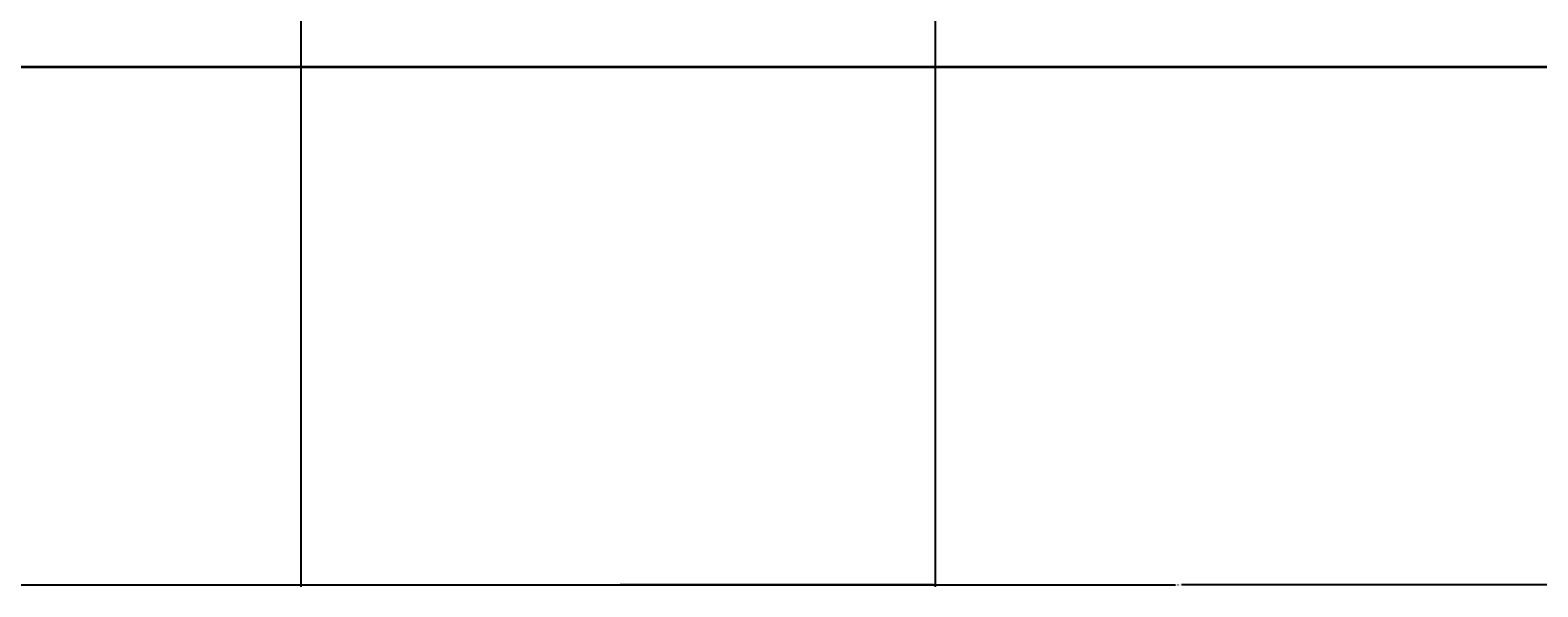
# Model space of a CAD drawing. Units: inches. Extents: x 3731 to 4318, y 1310 to 2388.
# Tile 8 of 57: x 3944 to 4086, y 1310 to 1363. Entities that reach past the tile are written whole.
import ezdxf

# ---------------------------------------------------------------- set-up
doc = ezdxf.new("R2010")
doc.units = ezdxf.units.IN
doc.layers.add('A-ANNO-DIMS', color=2, linetype='Continuous', lineweight=18)
doc.layers.add('A-WALL', color=7, linetype='Continuous', lineweight=35)
doc.styles.get("Standard").update_dxf_attribs({"font": 'arial.ttf'})
doc.dimstyles.get("Standard").update_dxf_attribs({"dimtxt": 0.18, "dimasz": 0.18, "dimexe": 0.18, "dimexo": 0.0625, "dimgap": 0.09, "dimtad": 0, "dimtih": 1, "dimtoh": 1, "dimdec": 4, "dimzin": 0, "dimdsep": 46, "dimtxsty": 'Standard', "dimcen": 0.09, "dimadec": 0, "dimazin": 0, "dimtfac": 1, "dimtdec": 4, "dimtofl": 0, "dimtmove": 0, "dimatfit": 3, "dimfxl": 1, "dimtolj": 1, "dimtzin": 0, "dimarcsym": 0})

# ---------------------------------------------------------------- blocks, each defined once
blk = doc.blocks.new('*D32')
at = {"layer": 'A-ANNO-DIMS', "color": 0, "lineweight": -2, "transparency": 16777216}
for p, q in [((4269.21, 1592.32), (4269.21, 1310.25)), ((3835.21, 1359.32), (3835.21, 1310.25)), ((3835.39, 1310.43), (4051.92, 1310.43)), ((4269.03, 1310.43), (4052.5, 1310.43))]:
    blk.add_line(p, q, dxfattribs=at)
at = {"layer": 'A-ANNO-DIMS', "color": 0, "transparency": 16777216}
for points in [[(3835.39, 1310.46), (3835.39, 1310.4), (3835.21, 1310.43)], [(4269.03, 1310.46), (4269.03, 1310.4), (4269.21, 1310.43)]]:
    blk.add_solid(points, dxfattribs=at)
at = {"layer": 'Defpoints', "color": 0, "transparency": 16777216}
for p in [(4269.21, 1592.38), (3835.21, 1359.38), (4269.21, 1310.43)]:
    blk.add_point(p, dxfattribs=at)
at = {"layer": 'A-ANNO-DIMS', "color": 0, "transparency": 16777216, "insert": (4052.21, 1310.43), "char_height": 0.18, "attachment_point": 5}
blk.add_mtext('\\A1;434', dxfattribs=at)
blk = doc.blocks.new('*D44')
at = {"layer": 'A-ANNO-DIMS', "color": 0, "lineweight": -2, "transparency": 16777216}
for p, q in [((3969.21, 1874.32), (3969.21, 1310.25)), ((4029.21, 1874.32), (4029.21, 1310.25)), ((3969.39, 1310.43), (3998.99, 1310.43)), ((4029.03, 1310.43), (3999.43, 1310.43))]:
    blk.add_line(p, q, dxfattribs=at)
at = {"layer": 'A-ANNO-DIMS', "color": 0, "transparency": 16777216}
for points in [[(3969.39, 1310.46), (3969.39, 1310.4), (3969.21, 1310.43)], [(4029.03, 1310.46), (4029.03, 1310.4), (4029.21, 1310.43)]]:
    blk.add_solid(points, dxfattribs=at)
at = {"layer": 'Defpoints', "color": 0, "transparency": 16777216}
for p in [(3969.21, 1874.38), (4029.21, 1874.38), (4029.21, 1310.43)]:
    blk.add_point(p, dxfattribs=at)
at = {"layer": 'A-ANNO-DIMS', "color": 0, "transparency": 16777216, "insert": (3999.21, 1310.43), "char_height": 0.18, "attachment_point": 5}
blk.add_mtext('\\A1;60', dxfattribs=at)

msp = doc.modelspace()

# ---------------------------------------------------------------- linework, layer by layer
at = {"layer": 'A-WALL'}
msp.add_line((3942.21, 1359.38), (4239.21, 1359.38), dxfattribs=at)

# ---------------------------------------------------------------- dimensions: what is measured, and where the dimension line sits
at = {"layer": 'A-ANNO-DIMS'}
for base, p1, p2, picture, middle in [((4029.21, 1310.43), (3969.21, 1874.38), (4029.21, 1874.38), '*D44', (3999.21, 1310.43)), ((4269.21, 1310.43), (3835.21, 1359.38), (4269.21, 1592.38), '*D32', (4052.21, 1310.43))]:
    dim = msp.add_linear_dim(base=base, p1=p1, p2=p2, dimstyle='Standard', override={"dimdec": 0, "dimlfac": 1, "dimrnd": 0, "dimzin": 0, "dimdsep": 46, "dimlunit": 2}, dxfattribs=at)
    dim.commit()
    dim.dimension.update_dxf_attribs({"geometry": picture, "text_midpoint": middle})

doc.saveas('drawing.dxf')
